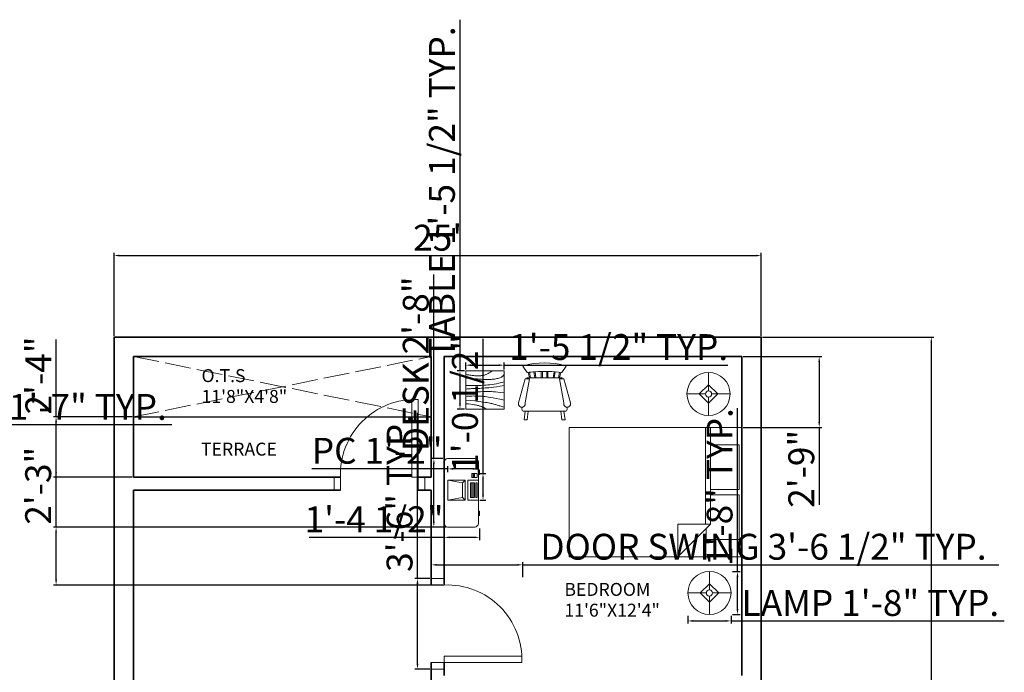
# Model space of a CAD drawing. Units: inches. Extents: x 2446 to 3341, y 462 to 1195.
# Tile 6 of 6: x 2884 to 3341, y 892 to 1195. Entities that reach past the tile are written whole.
import ezdxf

# ---------------------------------------------------------------- set-up
doc = ezdxf.new("R2010")
doc.units = ezdxf.units.IN
doc.linetypes.add('ACAD_ISO02W100', pattern=[15, 12, -3])
for name, color, linetype, lineweight in [('A-ANNO-DIMS', 2, 'Continuous', 18), ('A-AREA-IDEN', 7, 'Continuous', 18), ('A-DOOR', 4, 'Continuous', 18), ('A-EQPM', 9, 'Continuous', 18), ('A-FLOR', 7, 'Continuous', 25), ('A-FLOR-OPEN', 8, 'ACAD_ISO02W100', 13), ('A-FURN', 8, 'Continuous', 18), ('A-WALL', 7, 'Continuous', 35), ('C-PROP', 7, 'Continuous', 35)]:
    doc.layers.add(name, color=color, linetype=linetype, lineweight=lineweight)
doc.styles.get("Standard").update_dxf_attribs({"font": 'arial.ttf'})
doc.dimstyles.new('ISO-25', dxfattribs={"dimtxt": 12, "dimasz": 2.5, "dimexe": 1.25, "dimexo": 0.625, "dimtad": 1, "dimdec": 1, "dimlunit": 3, "dimtxsty": 'Standard', "dimcen": 2.5, "dimadec": 0, "dimazin": 0, "dimtfac": 1, "dimtdec": 1, "dimtmove": 0, "dimatfit": 3, "dimfxl": 1, "dimarcsym": 0})

# ---------------------------------------------------------------- blocks, each defined once
blk = doc.blocks.new('Desk - 30 x 60 in.')
for p, q in [((-26.999995, 0), (26.999995, 0)), ((-29.999995, -27), (-29.999995, -3)), ((29.999995, -3), (29.999995, -27)), ((26.999995, -30), (-26.999995, -30)), ((-20.000005, -30), (-20.000005, -31)), ((-20.000005, -31), (-16.000005, -31)), ((-16.000005, -31), (-16.000005, -30)), ((15.999995, -31), (15.999995, -30)), ((19.999995, -31), (15.999995, -31)), ((19.999995, -30), (19.999995, -31))]:
    blk.add_line(p, q)
for centre, start, end in [((-26.499995, -3.5), 98.1301, 171.8699), ((26.499995, -3.5), 8.130102, 81.8699), ((-26.499995, -26.5), 188.1301, 261.8699), ((26.499995, -26.5), 278.1301, 351.8699)]:
    blk.add_arc(centre, 3.535534, start, end)
blk = doc.blocks.new('Computer Terminal')
for p, q in [((-10, 11.5), (5, 11.5)), ((-8, 0.5), (-10, 11.5)), ((-10, -1.5), (-10, 11.5)), ((5, 11.5), (3, 0.5)), ((5, 11.5), (5, -1.5)), ((-10, -1.5), (-8, 0.5)), ((3, 0.5), (-8, 0.5)), ((3, 0.5), (5, -1.5)), ((5, -1.5), (-10, -1.5)), ((-10, -11.5), (-10, -3.5)), ((-10, -3.5), (5, -3.5)), ((-8, -5.5), (-8, -8.5)), ((3, -5.5), (-8, -5.5)), ((3, -6.5), (-8, -6.5)), ((3, -8.5), (3, -5.5)), ((5, -3.5), (5, -11.5)), ((10, -6.5), (7, -6.5)), ((7, -6.5), (7, -10.5)), ((10, -10.5), (10, -6.5)), ((5, -11.5), (-10, -11.5)), ((-8, -7.5), (3, -7.5)), ((-8, -8.5), (3, -8.5)), ((-8, -9.5), (-8, -10.5)), ((3, -9.5), (-8, -9.5)), ((-8, -10.5), (3, -10.5)), ((3, -10.5), (3, -9.5)), ((7, -10.5), (10, -10.5)), ((9.5, -7.5), (7.5, -7.5)), ((7.5, -7.5), (7.5, -8.5)), ((7.5, -8.5), (9.5, -8.5)), ((8.5, -7.5), (8.5, -8.5)), ((9.5, -8.5), (9.5, -7.5))]:
    blk.add_line(p, q)
blk = doc.blocks.new('Chair - Rocking')
for p, q in [((-8, -4.5), (-10, -1.5)), ((-7.5, -4.5), (-7, -7)), ((-6.5, -7), (-7.02225, -4.43)), ((-4.5, -7), (-4.96674, -4.19951)), ((-4, -7), (-4.40532, -4.16272)), ((-1.5, -4.05012), (-1.5, -7)), ((-1, -7), (-1, -4.05012)), ((1, -7), (1, -4.04655)), ((1.5, -4.05012), (1.5, -7)), ((4, -7), (4.40187, -4.18694)), ((4.5, -7), (4.96761, -4.19437)), ((6.5, -7), (7, -4.4057)), ((7.5, -4.5), (7, -7)), ((8, -4.5), (10, -1.5)), ((-9, -7.5), (-12, -18.49999)), ((-7, -7.5), (-9, -7.5)), ((-9, -18.49999), (-7, -7.5)), ((-8.23428, -6.99939), (-8.3093, -7.47958)), ((-8.23041, -7), (8.23915, -7)), ((7, -7.5), (9, -7.5)), ((9, -18.49999), (7, -7.5)), ((8.31071, -7.48854), (8.23449, -7.00073)), ((9, -7.5), (12, -18.49999)), ((-10.36644, -20.64523), (-10.5, -21.49999)), ((-9, -22.49999), (-9.5, -26.49999)), ((0, -22.49999), (-9.5, -22.49999)), ((-8, -26.49999), (-7.5, -22.49999)), ((0, -22.49999), (9.5, -22.49999)), ((8, -26.49999), (7.5, -22.49999)), ((9, -22.49999), (9.5, -26.49999)), ((10.5, -21.49999), (10.3575, -20.58798)), ((-9.5, -26.49999), (-8, -26.49999)), ((9.5, -26.49999), (8, -26.49999))]:
    blk.add_line(p, q)
for centre, radius, start, end in [((0, -34.08333), 34.08333, 72.93847, 107.0615), ((0, -68.25004), 64.25, 93.92211, 97.15267), ((0, -68.25004), 64.25, 82.84733, 93.92211), ((-10.5, -18.99999), 1.58114, 161.5651, 18.43495), ((-9.5, -21.49999), 1, 180, 270), ((10.5, -18.99999), 1.58114, 161.5651, 18.43495), ((9.5, -21.49999), 1, 270, 0)]:
    blk.add_arc(centre, radius, start, end)
blk = doc.blocks.new('Bed - Queen')
for p, q in [((0, -80.00003), (0, 0)), ((0, 0), (59.99999, 0)), ((59.99999, 0), (59.99999, -80.00003)), ((7.99999, -1.2), (28.79998, -1.2)), ((7.99999, -14.4), (7.99999, -1.2)), ((28.79998, -1.2), (28.79998, -14.4)), ((31.19999, -1.2), (51.99999, -1.2)), ((31.19999, -14.4), (31.19999, -1.2)), ((51.99999, -1.2), (51.99999, -16.4)), ((0, -14.4), (44.8, -14.4)), ((44.8, -16.8), (0, -16.8)), ((59.99999, -29.6), (44.8, -14.4)), ((44.8, -14.4), (44.8, -29.6)), ((51.99999, -16.4), (46.79936, -16.4)), ((44.8, -29.6), (59.99999, -29.6)), ((59.99999, -80.00003), (0, -80.00003))]:
    blk.add_line(p, q)
blk = doc.blocks.new('Lamp - Table')
for p, q in [((0, 7), (0, 1)), ((-1, 0), (-7, 0)), ((0, 3), (-3, 0)), ((-3, 0), (0, -3)), ((3, 0), (0, 3)), ((0, -3), (3, 0)), ((1, 0), (7, 0)), ((0, -1), (0, -7))]:
    blk.add_line(p, q)
for radius in [7, 1]:
    blk.add_circle((0, 0), radius)
blk = doc.blocks.new('Table - Square Woodgrain 42 x 42 in.')
blk.add_line((0, -42), (42, -42))
for points in [[(0, -4), (1.704, -4.2172), (3.2358, -4.4188), (4.615, -4.604), (5.8615, -4.7721), (6.9951, -4.9224), (8.0357, -5.0541), (9.0031, -5.1667), (9.9171, -5.2594), (10.7951, -5.3316), (11.6445, -5.3836), (12.4702, -5.4157), (13.277, -5.4283), (14.0698, -5.4217), (14.8535, -5.3964), (15.6331, -5.3526), (16.4133, -5.2908), (17.1986, -5.2103), (17.9913, -5.1062), (18.793, -4.9727), (19.6056, -4.8038), (20.4307, -4.5937), (21.2701, -4.3365), (22.1256, -4.0262), (22.9989, -3.6571), (23.888, -3.2272), (24.7756, -2.7516), (25.6408, -2.2491), (26.4624, -1.7387), (27.2195, -1.2395), (27.891, -0.7703), (28.456, -0.3501), (28.8934, 0.002)], [(0, -42), (0, 0), (42, 0), (42, -42)], [(0, -8), (1.8203, -8.1001), (3.6741, -8.2149), (5.5411, -8.3408), (7.4011, -8.4741), (9.2339, -8.6112), (11.0193, -8.7484), (12.7371, -8.8821), (14.3671, -9.0086), (15.8954, -9.1246), (17.3337, -9.2278), (18.6997, -9.3159), (20.0116, -9.387), (21.2871, -9.4389), (22.5442, -9.4696), (23.8008, -9.477), (25.0749, -9.459), (26.3791, -9.4137), (27.7049, -9.3403), (29.0383, -9.2382), (30.3655, -9.1068), (31.6728, -8.9455), (32.9461, -8.7535), (34.1717, -8.5304), (35.3358, -8.2756), (36.4268, -7.9863), (37.443, -7.6521), (38.3849, -7.2603), (39.253, -6.7986), (40.048, -6.2542), (40.7705, -5.6147), (41.421, -4.8674), (42, -4)], [(42, -12), (39.1784, -12.8621), (36.4519, -13.5654), (33.8246, -14.1294), (31.3004, -14.5731), (28.8832, -14.9161), (26.577, -15.1775), (24.3858, -15.3768), (22.3136, -15.5332), (20.3622, -15.6632), (18.5254, -15.7718), (16.7947, -15.8612), (15.1618, -15.9338), (13.6183, -15.9916), (12.1558, -16.0369), (10.7659, -16.0718), (9.4403, -16.0987), (8.1703, -16.1191), (6.9461, -16.1325), (5.7577, -16.1377), (4.595, -16.1335), (3.4479, -16.1188), (2.3064, -16.0924), (1.1604, -16.0532), (0, -16)], [(42, -16), (37.6529, -16.7365), (33.8802, -17.329), (30.6179, -17.7961), (27.8015, -18.1561), (25.3668, -18.4275), (23.2497, -18.6288), (21.3859, -18.7785), (19.7111, -18.8949), (18.1693, -18.9939), (16.7375, -19.0795), (15.401, -19.1534), (14.1449, -19.217), (12.9544, -19.2717), (11.8148, -19.3191), (10.7113, -19.3606), (9.6291, -19.3976), (8.5534, -19.4323), (7.47, -19.4689), (6.3643, -19.5122), (5.222, -19.5672), (4.0288, -19.6386), (2.7703, -19.7313), (1.4321, -19.8501), (0, -20)], [(0, -24), (3.9243, -23.6805), (7.4766, -23.4138), (10.6891, -23.1954), (13.5943, -23.0205), (16.2247, -22.8847), (18.6125, -22.7832), (20.7903, -22.7116), (22.7903, -22.6651), (24.6563, -22.642), (26.4764, -22.6507), (28.35, -22.7024), (30.3766, -22.8084), (32.6555, -22.98), (35.2861, -23.2283), (38.3678, -23.5645), (42, -24)], [(42, -32), (37.392, -31.017), (33.4585, -30.2231), (30.1291, -29.5949), (27.3334, -29.109), (25.0009, -28.742), (23.0612, -28.4707), (21.4439, -28.2716), (20.0786, -28.1215), (18.8998, -28.0002), (17.8609, -27.9014), (16.9206, -27.8219), (16.0371, -27.7588), (15.1691, -27.709), (14.2748, -27.6693), (13.3128, -27.6368), (12.2415, -27.6083), (11.0295, -27.5824), (9.6867, -27.5643), (8.233, -27.5608), (6.6884, -27.5787), (5.0728, -27.6248), (3.4062, -27.7058), (1.7086, -27.8286), (0, -28)], [(0, -32), (5.4026, -32.5358), (9.9494, -33.019), (13.7424, -33.4553), (16.8834, -33.8505), (19.4743, -34.2106), (21.6171, -34.5413), (23.4136, -34.8486), (24.9657, -35.1382), (26.3614, -35.4156), (27.6332, -35.6841), (28.7995, -35.9467), (29.8788, -36.2064), (30.8897, -36.4661), (31.8507, -36.7288), (32.7802, -36.9973), (33.6968, -37.2747), (34.6175, -37.5635), (35.5531, -37.8651), (36.5128, -38.1805), (37.506, -38.5108), (38.5421, -38.8568), (39.6302, -39.2197), (40.7797, -39.6004), (42, -40)], [(0, -36), (3.0098, -36.2857), (5.5354, -36.5643), (7.6368, -36.8359), (9.374, -37.1009), (10.807, -37.3597), (11.9957, -37.6126), (13.0002, -37.8599), (13.8804, -38.102), (14.6874, -38.3393), (15.4365, -38.5729), (16.1338, -38.8041), (16.7858, -39.0341), (17.3987, -39.264), (17.9787, -39.4952), (18.5322, -39.7288), (19.0655, -39.9662), (19.5832, -40.2081), (20.0842, -40.4544), (20.5657, -40.7046), (21.0249, -40.9581), (21.459, -41.2144), (21.8653, -41.4731), (22.2409, -41.7335), (22.5831, -41.9951)]]:
    blk.add_lwpolyline(points)
blk = doc.blocks.new('*D19')
at = {"layer": 'A-ANNO-DIMS', "color": 0, "lineweight": -2, "transparency": 16777216}
for p, q in [((2928.19, 1048.14), (2928.19, 1086.58)), ((3228.19, 1048.14), (3228.19, 1086.58)), ((2930.69, 1085.33), (3225.69, 1085.33))]:
    blk.add_line(p, q, dxfattribs=at)
at = {"layer": 'A-ANNO-DIMS', "color": 0, "transparency": 16777216}
for points in [[(2930.69, 1085.75), (2930.69, 1084.91), (2928.19, 1085.33)], [(3225.69, 1085.75), (3225.69, 1084.91), (3228.19, 1085.33)]]:
    blk.add_solid(points, dxfattribs=at)
at = {"layer": 'Defpoints', "color": 0, "transparency": 16777216}
for p in [(3228.19, 1085.33), (2928.19, 1047.51), (3228.19, 1047.51)]:
    blk.add_point(p, dxfattribs=at)
at = {"layer": 'A-ANNO-DIMS', "color": 0, "transparency": 16777216, "insert": (3078.19, 1092.08), "char_height": 12, "attachment_point": 5}
blk.add_mtext("25'", dxfattribs=at)
blk = doc.blocks.new('*D20')
at = {"layer": 'A-ANNO-DIMS', "color": 0, "lineweight": -2, "transparency": 16777216}
for p, q in [((3228.82, 1047.51), (3308.24, 1047.51)), ((3306.99, 1045.01), (3306.99, 570.01)), ((3228.82, 567.51), (3308.24, 567.51))]:
    blk.add_line(p, q, dxfattribs=at)
at = {"layer": 'A-ANNO-DIMS', "color": 0, "transparency": 16777216}
for points in [[(3306.57, 1045.01), (3307.4, 1045.01), (3306.99, 1047.51)], [(3306.57, 570.01), (3307.4, 570.01), (3306.99, 567.51)]]:
    blk.add_solid(points, dxfattribs=at)
at = {"layer": 'Defpoints', "color": 0, "transparency": 16777216}
for p in [(3228.19, 1047.51), (3228.19, 567.51), (3306.99, 567.51)]:
    blk.add_point(p, dxfattribs=at)
at = {"layer": 'A-ANNO-DIMS', "color": 0, "transparency": 16777216, "insert": (3300.24, 807.51), "char_height": 12, "attachment_point": 5, "rotation": 90}
blk.add_mtext("40'", dxfattribs=at)
blk = doc.blocks.new('DOOR-SWING-36IN')
for p, q in [((6, 42), (0, 42)), ((6, 39), (0, 39)), ((6, 3), (0, 3)), ((6, 0), (0, 0))]:
    blk.add_line(p, q)
blk.add_lwpolyline([(6, 3), (42, 3), (42, 6), (6, 6)], close=True)
blk.add_arc((7.5, 4.5), 34.53, 357.5104, 92.4896)
blk = doc.blocks.new('*D23')
at = {"layer": 'A-ANNO-DIMS', "color": 0, "lineweight": -2, "transparency": 16777216}
for p, q in [((3075.19, 936.14), (3075.19, 943.12)), ((3077.69, 941.87), (3115.11, 941.87)), ((3117.61, 936.14), (3117.61, 943.12)), ((3117.61, 941.87), (3338.29, 941.87))]:
    blk.add_line(p, q, dxfattribs=at)
at = {"layer": 'A-ANNO-DIMS', "color": 0, "transparency": 16777216}
for points in [[(3077.69, 942.29), (3077.69, 941.46), (3075.19, 941.87)], [(3115.11, 942.29), (3115.11, 941.46), (3117.61, 941.87)]]:
    blk.add_solid(points, dxfattribs=at)
at = {"layer": 'Defpoints', "color": 0, "transparency": 16777216}
for p in [(3117.61, 941.87), (3075.19, 935.51), (3117.61, 935.51)]:
    blk.add_point(p, dxfattribs=at)
at = {"layer": 'A-ANNO-DIMS', "color": 0, "transparency": 16777216, "insert": (3229.2, 948.71), "char_height": 12, "attachment_point": 5}
blk.add_mtext('DOOR SWING 3\'-6 1/2" TYP.', dxfattribs=at)
blk = doc.blocks.new('*D24')
at = {"layer": 'A-ANNO-DIMS', "color": 0, "lineweight": -2, "transparency": 16777216}
for p, q in [((3068.83, 935.51), (3068.83, 1012.4)), ((3074.57, 935.51), (3067.58, 935.51)), ((3068.83, 896.01), (3068.83, 933.01)), ((3074.57, 893.51), (3067.58, 893.51))]:
    blk.add_line(p, q, dxfattribs=at)
at = {"layer": 'A-ANNO-DIMS', "color": 0, "transparency": 16777216}
for points in [[(3068.41, 933.01), (3069.25, 933.01), (3068.83, 935.51)], [(3068.41, 896.01), (3069.25, 896.01), (3068.83, 893.51)]]:
    blk.add_solid(points, dxfattribs=at)
at = {"layer": 'Defpoints', "color": 0, "transparency": 16777216}
for p in [(3068.83, 935.51), (3075.19, 935.51), (3075.19, 893.51)]:
    blk.add_point(p, dxfattribs=at)
at = {"layer": 'A-ANNO-DIMS', "color": 0, "transparency": 16777216, "insert": (3062.08, 975.2), "char_height": 12, "attachment_point": 5, "rotation": 90}
blk.add_mtext('3\'-6" TYP.', dxfattribs=at)
blk = doc.blocks.new('*D25')
at = {"layer": 'A-ANNO-DIMS', "color": 0, "lineweight": -2, "transparency": 16777216}
for p, q in [((2809.62, 1009.12), (2809.62, 1005.68)), ((2828.38, 1009.12), (2828.38, 1005.68)), ((2812.12, 1006.93), (2825.88, 1006.93)), ((2828.38, 1006.93), (2955.05, 1006.93))]:
    blk.add_line(p, q, dxfattribs=at)
at = {"layer": 'A-ANNO-DIMS', "color": 0, "transparency": 16777216}
for points in [[(2812.12, 1007.35), (2812.12, 1006.52), (2809.62, 1006.93)], [(2825.88, 1007.35), (2825.88, 1006.52), (2828.38, 1006.93)]]:
    blk.add_solid(points, dxfattribs=at)
at = {"layer": 'Defpoints', "color": 0, "transparency": 16777216}
for p in [(2809.62, 1009.75), (2828.38, 1009.75), (2828.38, 1006.93)]:
    blk.add_point(p, dxfattribs=at)
at = {"layer": 'A-ANNO-DIMS', "color": 0, "transparency": 16777216, "insert": (2892.96, 1013.59), "char_height": 12, "attachment_point": 5}
blk.add_mtext('LAMP 1\'-7" TYP.', dxfattribs=at)
blk = doc.blocks.new('*D27')
at = {"layer": 'A-ANNO-DIMS', "color": 0, "lineweight": -2, "transparency": 16777216}
for p, q in [((3194.2, 918.23), (3194.2, 914.61)), ((3214.16, 918.23), (3214.16, 914.61)), ((3196.7, 915.86), (3211.66, 915.86)), ((3214.16, 915.86), (3340.83, 915.86))]:
    blk.add_line(p, q, dxfattribs=at)
at = {"layer": 'A-ANNO-DIMS', "color": 0, "transparency": 16777216}
for points in [[(3196.7, 916.27), (3196.7, 915.44), (3194.2, 915.86)], [(3211.66, 916.27), (3211.66, 915.44), (3214.16, 915.86)]]:
    blk.add_solid(points, dxfattribs=at)
at = {"layer": 'Defpoints', "color": 0, "transparency": 16777216}
for p in [(3194.2, 918.85), (3214.16, 918.85), (3214.16, 915.86)]:
    blk.add_point(p, dxfattribs=at)
at = {"layer": 'A-ANNO-DIMS', "color": 0, "transparency": 16777216, "insert": (3278.74, 922.61), "char_height": 12, "attachment_point": 5}
blk.add_mtext('LAMP 1\'-8" TYP.', dxfattribs=at)
blk = doc.blocks.new('*D28')
at = {"layer": 'A-ANNO-DIMS', "color": 0, "lineweight": -2, "transparency": 16777216}
for p, q in [((3217.15, 938.8), (3217.15, 1014.57)), ((3214.78, 938.8), (3218.4, 938.8)), ((3217.15, 921.35), (3217.15, 936.3)), ((3214.78, 918.85), (3218.4, 918.85))]:
    blk.add_line(p, q, dxfattribs=at)
at = {"layer": 'A-ANNO-DIMS', "color": 0, "transparency": 16777216}
for points in [[(3216.73, 936.3), (3217.57, 936.3), (3217.15, 938.8)], [(3216.73, 921.35), (3217.57, 921.35), (3217.15, 918.85)]]:
    blk.add_solid(points, dxfattribs=at)
at = {"layer": 'Defpoints', "color": 0, "transparency": 16777216}
for p in [(3214.16, 938.8), (3217.15, 938.8), (3214.16, 918.85)]:
    blk.add_point(p, dxfattribs=at)
at = {"layer": 'A-ANNO-DIMS', "color": 0, "transparency": 16777216, "insert": (3210.4, 977.94), "char_height": 12, "attachment_point": 5, "rotation": 90}
blk.add_mtext('1\'-8" TYP.', dxfattribs=at)
blk = doc.blocks.new('*D39')
at = {"layer": 'A-ANNO-DIMS', "color": 0, "lineweight": -2, "transparency": 16777216}
for p, q in [((3088.55, 1031.84), (3088.55, 1194.76)), ((3090.58, 1031.84), (3087.3, 1031.84)), ((3088.55, 1016.59), (3088.55, 1029.34)), ((3090.58, 1014.09), (3087.3, 1014.09))]:
    blk.add_line(p, q, dxfattribs=at)
at = {"layer": 'A-ANNO-DIMS', "color": 0, "transparency": 16777216}
for points in [[(3088.13, 1029.34), (3088.96, 1029.34), (3088.55, 1031.84)], [(3088.13, 1016.59), (3088.96, 1016.59), (3088.55, 1014.09)]]:
    blk.add_solid(points, dxfattribs=at)
at = {"layer": 'Defpoints', "color": 0, "transparency": 16777216}
for p in [(3088.55, 1031.84), (3091.21, 1031.84), (3091.21, 1014.09)]:
    blk.add_point(p, dxfattribs=at)
at = {"layer": 'A-ANNO-DIMS', "color": 0, "transparency": 16777216, "insert": (3081.72, 1114.55), "char_height": 12, "attachment_point": 5, "rotation": 90}
blk.add_mtext('TABLE 1\'-5 1/2" TYP.', dxfattribs=at)
blk = doc.blocks.new('*D40')
at = {"layer": 'A-ANNO-DIMS', "color": 0, "lineweight": -2, "transparency": 16777216}
for p, q in [((3091.21, 1032.46), (3091.21, 1035.75)), ((3093.71, 1034.5), (3106.46, 1034.5)), ((3108.96, 1032.46), (3108.96, 1035.75)), ((3108.96, 1034.5), (3212.68, 1034.5))]:
    blk.add_line(p, q, dxfattribs=at)
at = {"layer": 'A-ANNO-DIMS', "color": 0, "transparency": 16777216}
for points in [[(3093.71, 1034.92), (3093.71, 1034.08), (3091.21, 1034.5)], [(3106.46, 1034.92), (3106.46, 1034.08), (3108.96, 1034.5)]]:
    blk.add_solid(points, dxfattribs=at)
at = {"layer": 'Defpoints', "color": 0, "transparency": 16777216}
for p in [(3091.21, 1031.84), (3108.96, 1034.5), (3108.96, 1031.84)]:
    blk.add_point(p, dxfattribs=at)
at = {"layer": 'A-ANNO-DIMS', "color": 0, "transparency": 16777216, "insert": (3162.07, 1041.33), "char_height": 12, "attachment_point": 5}
blk.add_mtext('1\'-5 1/2" TYP.', dxfattribs=at)
blk = doc.blocks.new('*D43')
at = {"layer": 'A-ANNO-DIMS', "color": 0, "lineweight": -2, "transparency": 16777216}
for p, q in [((3076.43, 991.18), (3076.43, 1076.54)), ((3080.57, 991.18), (3075.18, 991.18)), ((3076.43, 961.89), (3076.43, 988.68)), ((3080.57, 959.39), (3075.18, 959.39))]:
    blk.add_line(p, q, dxfattribs=at)
at = {"layer": 'A-ANNO-DIMS', "color": 0, "transparency": 16777216}
for points in [[(3076.01, 988.68), (3076.84, 988.68), (3076.43, 991.18)], [(3076.01, 961.89), (3076.84, 961.89), (3076.43, 959.39)]]:
    blk.add_solid(points, dxfattribs=at)
at = {"layer": 'Defpoints', "color": 0, "transparency": 16777216}
for p in [(3076.43, 991.18), (3081.19, 991.18), (3081.19, 959.39)]:
    blk.add_point(p, dxfattribs=at)
at = {"layer": 'A-ANNO-DIMS', "color": 0, "transparency": 16777216, "insert": (3069.6, 1035.11), "char_height": 12, "attachment_point": 5, "rotation": 90}
blk.add_mtext('DESK 2\'-8"', dxfattribs=at)
blk = doc.blocks.new('*D44')
at = {"layer": 'A-ANNO-DIMS', "color": 0, "lineweight": -2, "transparency": 16777216}
for p, q in [((3081.19, 958.76), (3081.19, 953.37)), ((3097.62, 958.76), (3097.62, 953.37)), ((3081.19, 954.62), (3018.71, 954.62)), ((3095.12, 954.62), (3083.69, 954.62))]:
    blk.add_line(p, q, dxfattribs=at)
at = {"layer": 'A-ANNO-DIMS', "color": 0, "transparency": 16777216}
for points in [[(3083.69, 955.04), (3083.69, 954.2), (3081.19, 954.62)], [(3095.12, 955.04), (3095.12, 954.2), (3097.62, 954.62)]]:
    blk.add_solid(points, dxfattribs=at)
at = {"layer": 'Defpoints', "color": 0, "transparency": 16777216}
for p in [(3081.19, 959.39), (3097.62, 959.39), (3081.19, 954.62)]:
    blk.add_point(p, dxfattribs=at)
at = {"layer": 'A-ANNO-DIMS', "color": 0, "transparency": 16777216, "insert": (3048.7, 961.45), "char_height": 12, "attachment_point": 5}
blk.add_mtext('1\'-4 1/2"', dxfattribs=at)
blk = doc.blocks.new('*D47')
at = {"layer": 'A-ANNO-DIMS', "color": 0, "lineweight": -2, "transparency": 16777216}
for p, q in [((3082.89, 986.4), (3019.89, 986.4)), ((3082.89, 984.9), (3082.89, 987.65)), ((3094.59, 986.4), (3085.39, 986.4)), ((3097.09, 984.9), (3097.09, 987.65))]:
    blk.add_line(p, q, dxfattribs=at)
at = {"layer": 'A-ANNO-DIMS', "color": 0, "transparency": 16777216}
for points in [[(3085.39, 986.82), (3085.39, 985.98), (3082.89, 986.4)], [(3094.59, 986.82), (3094.59, 985.98), (3097.09, 986.4)]]:
    blk.add_solid(points, dxfattribs=at)
at = {"layer": 'Defpoints', "color": 0, "transparency": 16777216}
for p in [(3082.89, 986.4), (3082.89, 984.27), (3097.09, 984.27)]:
    blk.add_point(p, dxfattribs=at)
at = {"layer": 'A-ANNO-DIMS', "color": 0, "transparency": 16777216, "insert": (3050.14, 993.23), "char_height": 12, "attachment_point": 5}
blk.add_mtext('PC 1\'-2"', dxfattribs=at)
blk = doc.blocks.new('*D48')
at = {"layer": 'A-ANNO-DIMS', "color": 0, "lineweight": -2, "transparency": 16777216}
for p, q in [((3099.22, 984.27), (3099.22, 1046.75)), ((3097.71, 984.27), (3100.47, 984.27)), ((3099.22, 974.42), (3099.22, 981.77)), ((3097.71, 971.92), (3100.47, 971.92))]:
    blk.add_line(p, q, dxfattribs=at)
at = {"layer": 'A-ANNO-DIMS', "color": 0, "transparency": 16777216}
for points in [[(3098.8, 981.77), (3099.64, 981.77), (3099.22, 984.27)], [(3098.8, 974.42), (3099.64, 974.42), (3099.22, 971.92)]]:
    blk.add_solid(points, dxfattribs=at)
at = {"layer": 'Defpoints', "color": 0, "transparency": 16777216}
for p in [(3097.09, 984.27), (3099.22, 984.27), (3097.09, 971.92)]:
    blk.add_point(p, dxfattribs=at)
at = {"layer": 'A-ANNO-DIMS', "color": 0, "transparency": 16777216, "insert": (3092.39, 1016.76), "char_height": 12, "attachment_point": 5, "rotation": 90}
blk.add_mtext('1\'-0 1/2"', dxfattribs=at)
blk = doc.blocks.new('*D64')
at = {"layer": 'A-ANNO-DIMS', "color": 0, "lineweight": -2, "transparency": 16777216}
for p, q in [((2901.34, 1010.51), (2901.34, 1046.36)), ((2936.57, 1010.51), (2900.09, 1010.51)), ((2901.34, 985.01), (2901.34, 1008.01)), ((2936.57, 982.51), (2900.09, 982.51))]:
    blk.add_line(p, q, dxfattribs=at)
at = {"layer": 'A-ANNO-DIMS', "color": 0, "transparency": 16777216}
for points in [[(2900.93, 1008.01), (2901.76, 1008.01), (2901.34, 1010.51)], [(2900.93, 985.01), (2901.76, 985.01), (2901.34, 982.51)]]:
    blk.add_solid(points, dxfattribs=at)
at = {"layer": 'Defpoints', "color": 0, "transparency": 16777216}
for p in [(2901.34, 1010.51), (2937.19, 1010.51), (2937.19, 982.51)]:
    blk.add_point(p, dxfattribs=at)
at = {"layer": 'A-ANNO-DIMS', "color": 0, "transparency": 16777216, "insert": (2894.69, 1029.69), "char_height": 12, "attachment_point": 5, "rotation": 90}
blk.add_mtext('2\'-4"', dxfattribs=at)
blk = doc.blocks.new('*D76')
at = {"layer": 'A-ANNO-DIMS', "color": 0, "lineweight": -2, "transparency": 16777216}
for p, q in [((3219.82, 1038.51), (3256.29, 1038.51)), ((3255.04, 1036.01), (3255.04, 1008.09)), ((3219.75, 1005.59), (3256.29, 1005.59)), ((3255.04, 1005.59), (3255.04, 969.74))]:
    blk.add_line(p, q, dxfattribs=at)
at = {"layer": 'A-ANNO-DIMS', "color": 0, "transparency": 16777216}
for points in [[(3254.63, 1036.01), (3255.46, 1036.01), (3255.04, 1038.51)], [(3254.63, 1008.09), (3255.46, 1008.09), (3255.04, 1005.59)]]:
    blk.add_solid(points, dxfattribs=at)
at = {"layer": 'Defpoints', "color": 0, "transparency": 16777216}
for p in [(3219.19, 1038.51), (3219.12, 1005.59), (3255.04, 1005.59)]:
    blk.add_point(p, dxfattribs=at)
at = {"layer": 'A-ANNO-DIMS', "color": 0, "transparency": 16777216, "insert": (3248.29, 986.42), "char_height": 12, "attachment_point": 5, "rotation": 90}
blk.add_mtext('2\'-9"', dxfattribs=at)
blk = doc.blocks.new('*D78')
at = {"layer": 'A-ANNO-DIMS', "color": 0, "lineweight": -2, "transparency": 16777216}
for p, q in [((2901.34, 959.39), (2901.34, 995.24)), ((3082.16, 959.39), (2900.09, 959.39)), ((2901.34, 935.01), (2901.34, 956.89)), ((3080.57, 932.51), (2900.09, 932.51))]:
    blk.add_line(p, q, dxfattribs=at)
at = {"layer": 'A-ANNO-DIMS', "color": 0, "transparency": 16777216}
for points in [[(2900.93, 956.89), (2901.76, 956.89), (2901.34, 959.39)], [(2900.93, 935.01), (2901.76, 935.01), (2901.34, 932.51)]]:
    blk.add_solid(points, dxfattribs=at)
at = {"layer": 'Defpoints', "color": 0, "transparency": 16777216}
for p in [(2901.34, 959.39), (3082.78, 959.39), (3081.19, 932.51)]:
    blk.add_point(p, dxfattribs=at)
at = {"layer": 'A-ANNO-DIMS', "color": 0, "transparency": 16777216, "insert": (2894.59, 978.57), "char_height": 12, "attachment_point": 5, "rotation": 90}
blk.add_mtext('2\'-3"', dxfattribs=at)

msp = doc.modelspace()

# ---------------------------------------------------------------- linework, layer by layer
at = {"layer": 'A-FLOR'}
msp.add_line((2937.19, 1010.51), (3075.19, 1010.51), dxfattribs=at)
at = {"layer": 'A-FLOR-OPEN'}
for p, q in [((2937.19, 1038.51), (3075.19, 1010.51)), ((2937.19, 1010.51), (3075.19, 1038.51))]:
    msp.add_line(p, q, dxfattribs=at)
at = {"layer": 'A-WALL'}
for p, q in [((2937.19, 1038.51), (2937.19, 982.51)), ((3075.19, 1038.51), (2937.19, 1038.51)), ((3075.19, 982.51), (3075.19, 1038.51)), ((3219.19, 1038.51), (3081.19, 1038.51)), ((3081.19, 932.51), (3081.19, 1038.51)), ((3219.19, 890.51), (3219.19, 1038.51)), ((3033.19, 982.51), (2937.19, 982.51)), ((3075.19, 982.51), (3069.19, 982.51)), ((2937.19, 976.51), (2937.19, 762.51)), ((3033.19, 976.51), (2937.19, 976.51)), ((3075.19, 976.51), (3069.19, 976.51)), ((3075.19, 932.51), (3075.19, 976.51)), ((3075.19, 884.51), (3075.19, 896.51)), ((3081.19, 890.51), (3081.19, 896.51))]:
    msp.add_line(p, q, dxfattribs=at)
at = {"layer": 'C-PROP'}
msp.add_lwpolyline([(3219.19, 567.51), (3228.19, 567.51), (3228.19, 1047.51), (2928.19, 1047.51), (2928.19, 567.51), (3219.19, 567.51)], dxfattribs=at)

# ---------------------------------------------------------------- block references
at = {"layer": 'A-DOOR', "rotation": 89.99999999999841}
msp.add_blockref('DOOR-SWING-36IN', (3072.19, 976.51), dxfattribs=at)
at = {"layer": 'A-DOOR'}
msp.add_blockref('DOOR-SWING-36IN', (3075.19, 893.51), dxfattribs=at)
at = {"layer": 'A-EQPM', "xscale": 0.6175466263156437, "yscale": 0.6175466263156437, "zscale": 0.6175466263156437, "rotation": 90}
msp.add_blockref('Computer Terminal', (3089.99, 978.09), dxfattribs=at)
at = {"layer": 'A-FURN'}
msp.add_blockref('Chair - Rocking', (3127.72, 1035.58), dxfattribs=at)
for name, p, xscale, yscale, zscale in [('Table - Square Woodgrain 42 x 42 in.', (3091.21, 1031.84), 0.4225793385240015, 0.4225793385240015, 0.4225793385240015), ('Lamp - Table', (3203.73, 1021.13), 1.425214435139041, 1.425214435139041, 1.425214435139041), ('Lamp - Table', (3204.18, 928.83), 1.425214435139041, 1.425214435139041, 1.425214435139041)]:
    msp.add_blockref(name, p, dxfattribs=dict(at, xscale=xscale, yscale=yscale, zscale=zscale))
at = {"layer": 'A-FURN', "rotation": 270}
msp.add_blockref('Bed - Queen', (3219.12, 1005.59), dxfattribs=at)
at = {"layer": 'A-FURN', "xscale": 0.5298361459739285, "yscale": 0.5298361459739285, "zscale": 0.5298361459739285, "rotation": 90}
msp.add_blockref('Desk - 30 x 60 in.', (3081.19, 975.28), dxfattribs=at)

# ---------------------------------------------------------------- texts
at = {"layer": 'A-AREA-IDEN'}
for s, p in [('O.T.S', (2968.74, 1026.64)), ('11\'8"X4\'8"', (2968.74, 1017)), ('TERRACE', (2968.51, 992.54)), ('BEDROOM', (3136.93, 927.48)), ('11\'6"X12\'4"', (3136.93, 917.84))]:
    msp.add_text(s, height=6, dxfattribs=at).set_placement(p)

# ---------------------------------------------------------------- dimensions: what is measured, and where the dimension line sits
at = {"layer": 'A-ANNO-DIMS'}
for base, p1, p2, angle, text, picture, middle in [((3088.5457, 1031.836), (3091.208, 1014.0868), (3091.208, 1031.836), 90, 'TABLE <> TYP.', '*D39', (3081.716, 1114.549)), ((3076.43, 991.18), (3081.19, 959.39), (3081.19, 991.18), 90, 'DESK <>', '*D43', (3069.6, 1035.11)), ((3217.1497, 938.8035), (3214.1567, 918.8505), (3214.1567, 938.8035), 90, '<> TYP.', '*D28', (3210.3978, 977.9367)), ((3082.89, 986.4), (3097.09, 984.27), (3082.89, 984.27), 180, 'PC <>', '*D47', (3050.14, 993.23)), ((3068.83, 935.51), (3075.19, 893.51), (3075.19, 935.51), 90, '<> TYP.', '*D24', (3062.08, 975.2))]:
    dim = msp.add_linear_dim(base=base, p1=p1, p2=p2, angle=angle, text=text, dimstyle='ISO-25', override={"dimdec": 1, "dimlfac": 1, "dimrnd": 0, "dimzin": 1, "dimdsep": 46, "dimlunit": 4, "dimfrac": 2}, dxfattribs=at)
    dim.commit()
    dim.dimension.update_dxf_attribs({"geometry": picture, "text_midpoint": middle})
dim = msp.add_linear_dim(base=(3228.19, 1085.33), p1=(2928.19, 1047.51), p2=(3228.19, 1047.51), dimstyle='ISO-25', override={"dimclrd": 0, "dimclre": 0, "dimclrt": 0}, dxfattribs=at)
dim.commit()
dim.dimension.update_dxf_attribs({"geometry": '*D19', "text_midpoint": (3078.19, 1092.08)})
for base, p1, p2, text, picture, middle in [((3108.9564, 1034.4984), (3091.208, 1031.836), (3108.9564, 1031.836), '<> TYP.', '*D40', (3162.0705, 1041.328)), ((2828.38, 1006.93), (2809.62, 1009.75), (2828.38, 1009.75), 'LAMP <> TYP.', '*D25', (2892.96, 1013.59)), ((3117.61, 941.87), (3075.19, 935.51), (3117.61, 935.51), 'DOOR SWING <> TYP.', '*D23', (3229.2, 948.71)), ((3214.16, 915.86), (3194.2, 918.85), (3214.16, 918.85), 'LAMP <> TYP.', '*D27', (3278.74, 922.61))]:
    dim = msp.add_linear_dim(base=base, p1=p1, p2=p2, text=text, dimstyle='ISO-25', override={"dimdec": 1, "dimlfac": 1, "dimrnd": 0, "dimzin": 1, "dimdsep": 46, "dimlunit": 4, "dimfrac": 2}, dxfattribs=at)
    dim.commit()
    dim.dimension.update_dxf_attribs({"geometry": picture, "text_midpoint": middle})
for base, p1, p2, angle, override, picture, middle in [((2901.34, 1010.51), (2937.19, 982.51), (2937.19, 1010.51), 90, {"dimdec": 1, "dimlfac": 1, "dimrnd": 0, "dimzin": 1, "dimdsep": 46, "dimlunit": 4, "dimfrac": 2}, '*D64', (2894.69, 1029.69)), ((3099.2201, 984.2703), (3097.0895, 971.9194), (3097.0895, 984.2703), 90, {"dimdec": 1, "dimlfac": 1, "dimrnd": 0, "dimzin": 1, "dimdsep": 46, "dimlunit": 4, "dimfrac": 2}, '*D48', (3092.3904, 1016.7609)), ((3306.99, 567.51), (3228.19, 1047.51), (3228.19, 567.51), 90, {"dimclrd": 0, "dimclre": 0, "dimclrt": 0}, '*D20', (3300.24, 807.51)), ((3255.04, 1005.59), (3219.19, 1038.51), (3219.12, 1005.59), 90, {"dimdec": 1, "dimlfac": 1, "dimrnd": 0, "dimzin": 1, "dimdsep": 46, "dimlunit": 4, "dimfrac": 2}, '*D76', (3248.29, 986.42)), ((2901.34, 959.39), (3081.19, 932.51), (3082.78, 959.39), 90, {"dimdec": 1, "dimlfac": 1, "dimrnd": 0, "dimzin": 1, "dimdsep": 46, "dimlunit": 4, "dimfrac": 2}, '*D78', (2894.59, 978.57)), ((3081.19, 954.62), (3097.62, 959.39), (3081.19, 959.39), 180, {"dimdec": 1, "dimlfac": 1, "dimrnd": 0, "dimzin": 1, "dimdsep": 46, "dimlunit": 4, "dimfrac": 2}, '*D44', (3048.7, 961.45))]:
    dim = msp.add_linear_dim(base=base, p1=p1, p2=p2, angle=angle, dimstyle='ISO-25', override=override, dxfattribs=at)
    dim.commit()
    dim.dimension.update_dxf_attribs({"geometry": picture, "text_midpoint": middle})

doc.saveas('drawing.dxf')
